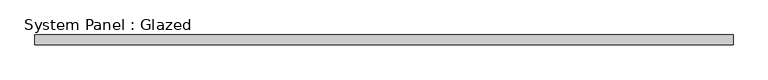
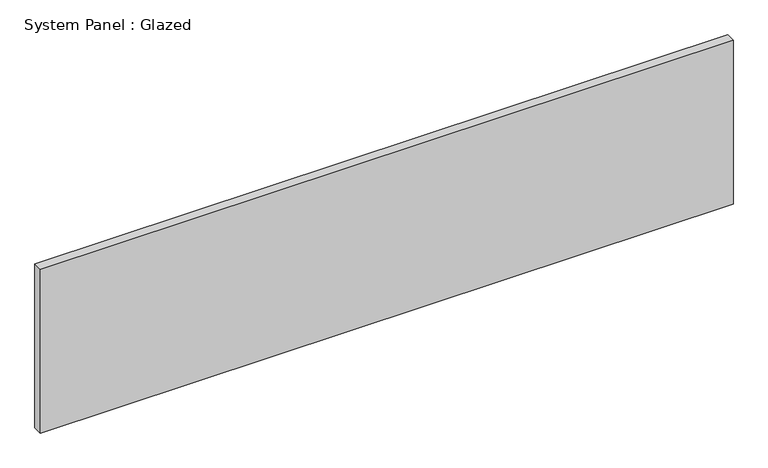
"""IFC4 building model written with IfcOpenShell, lengths in millimetres: plate geometry, System Panel : Glazed."""

from ifc_helpers import new_model, si_unit, origin, origin_with_axes, place, context, project, spatial, polyline, outline, extrude, source, transform, mapped, element, save


def system_panel_glazed_f05af352(model_context):
    return source(origin(), model_context, "Body", "SweptSolid", [
        extrude(outline(polyline([(914.4000002, -44.45), (-914.4000002, -44.45), (-914.4000002, -19.05), (914.4000002, -19.05), (914.4000002, -44.45)])), origin_with_axes(), (0.0, 0.0, 1.0), 457.2),
    ])


if __name__ == "__main__":
    model = new_model("IFC4")
    model_context = context("Model", 3, world=origin())
    ifc_project = project(units=[si_unit("LENGTHUNIT", "METRE", prefix="MILLI")], contexts=[model_context])
    site = spatial("IfcSite", under=ifc_project)
    building = spatial("IfcBuilding", under=site)
    placement = place(None, origin())
    system_panel_glazed_shape = system_panel_glazed_f05af352(model_context)
    element("IfcPlate", 1, ObjectType="System Panel : Glazed", at=placement, inside=building, context=model_context, shape_type="MappedRepresentation", body=[
        mapped(system_panel_glazed_shape, transform((0.0, 0.0, 0.0), x_axis=(1.0, 0.0, 0.0), y_axis=(0.0, 1.0, 0.0), z_axis=(0.0, 0.0, 1.0))),
    ])
    save(model, "model.ifc")

# Revit data of these elements
# Type "System Panel : Glazed"
#   Construction Type Id = "GSP4R"
#   Analytic Construction = "1/8 in Pilkington single glazing"
#   Visual Light Transmittance = 0.9
#   Solar Heat Gain Coefficient = 0.86
#   Heat Transfer Coefficient (U) = 1.18115 BTU/(h·ft²·°F)
#   Define Thermal Properties by = 1
# Element 1 (IfcPlate, "System Panel : Glazed")
#   Materials on its faces: "Glass"
# Materials
#   "Glass": class "Glass", colour RGB 0 128 192, transparency 0.75, Description = "Soda Lime Glass", Cost = 0
